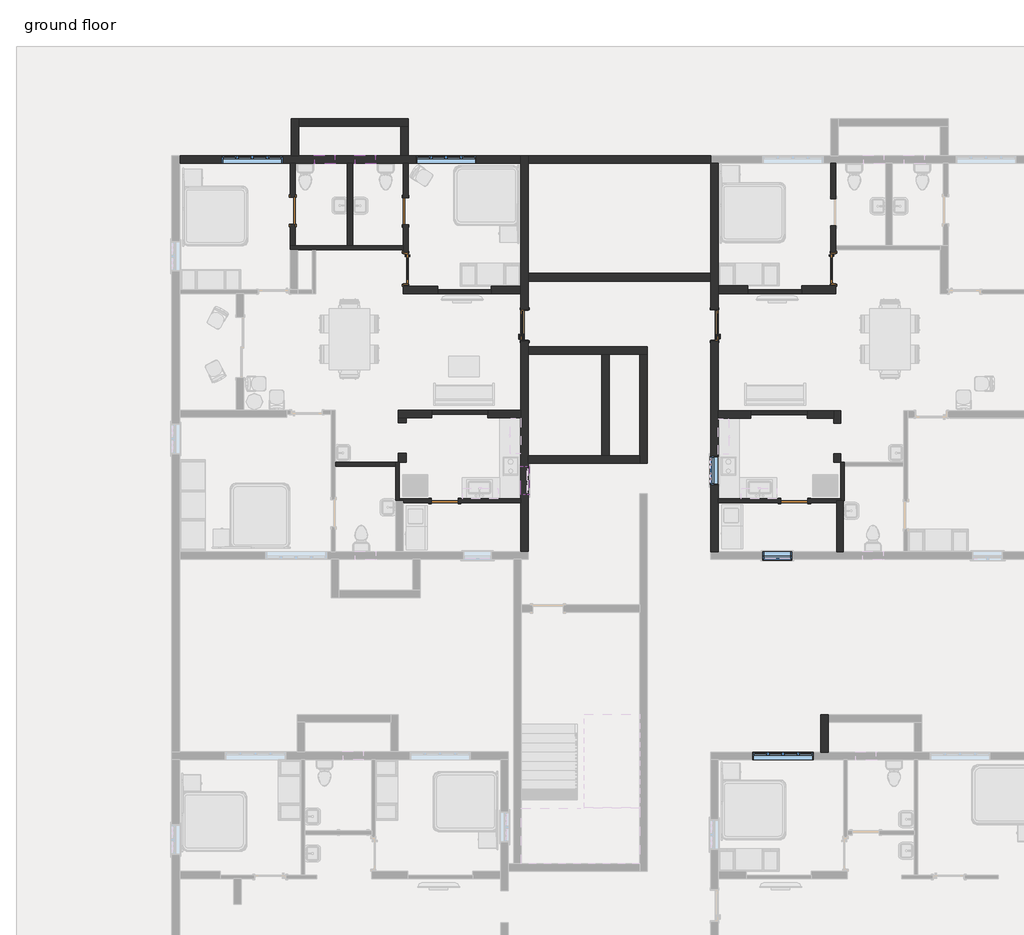
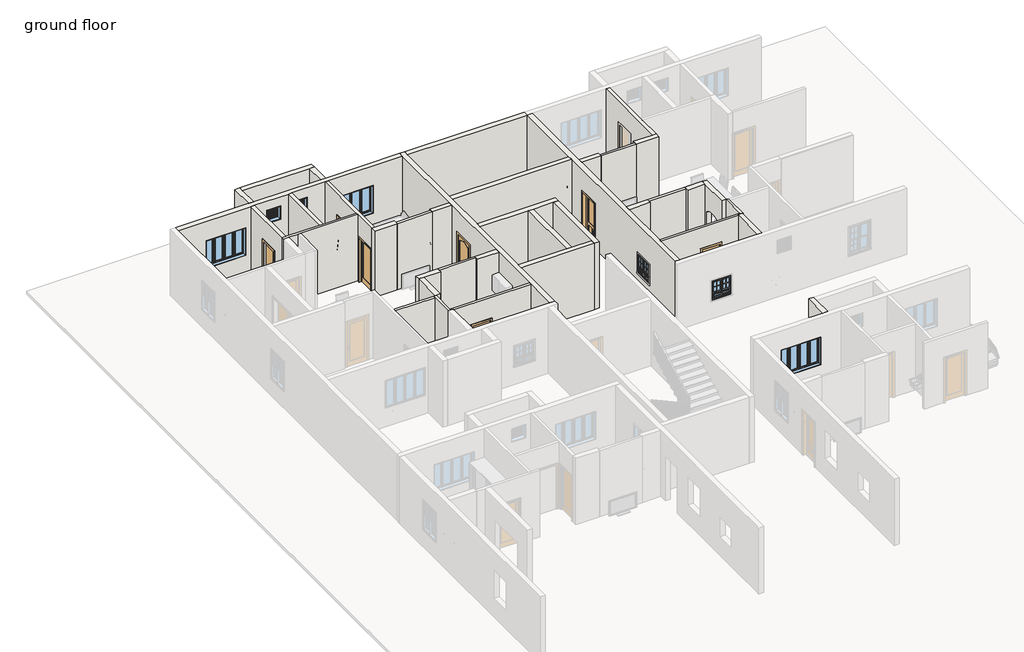
# One storey, part 8 of 16: 38 walls, 8 doors, 8 windows.
"""IFC4 building model written with IfcOpenShell, lengths in millimetres."""

from ifc_helpers import new_model, si_unit, point, frame, origin, place, context, project, spatial, polyline, ellipse_curve, trimmed, outline, extrude, faceted_brep, transform, mapped, element, save
from ifc_brep_helpers import plane_surface, extruded_surface, advanced_brep
from components import door_fe8ae985, door_f079f64e, door_010cc4d9, door_5a860750, door_377e7377, door_bb092f7c, door_38851409, door_d141acb4, window_ced37e8f, window_5487fb6d, window_f2d8fef0

model = new_model("IFC4")

# Units and contexts
model_context = context("Model", 3, world=origin())
ifc_project = project(units=[si_unit("LENGTHUNIT", "METRE", prefix="MILLI")], contexts=[model_context])

# Site, building, storey
site = spatial("IfcSite", under=ifc_project)
building = spatial("IfcBuilding", under=site)
storey = spatial("IfcBuildingStorey", under=building, Name="ground floor", Elevation=609.6)

# Doors
placement = place(None, origin())
door_shape = door_fe8ae985(model_context)
element("IfcDoor", 1, ObjectType="36\" x 84\"", at=placement, inside=storey, context=model_context, shape_type="MappedRepresentation", body=[
    mapped(door_shape, transform((53752.6562819, 45481.1632967, 609.6), x_axis=(0.0, -1.0, 0.0), y_axis=(1.0, 0.0, 0.0), z_axis=(0.0, 0.0, 1.0))),
])
door_2_shape = door_f079f64e(model_context)
element("IfcDoor", 2, ObjectType="36\" x 84\"", at=placement, inside=storey, context=model_context, shape_type="MappedRepresentation", body=[
    mapped(door_2_shape, transform((59474.0062819, 45484.6897902, 609.6), x_axis=(0.0, -1.0, 0.0), y_axis=(1.0, 0.0, 0.0), z_axis=(0.0, 0.0, 1.0))),
])
door_3_shape = door_010cc4d9(model_context)
element("IfcDoor", 3, ObjectType="Door-Interior-Single-1_Panel-Wood : 36\" x 84\"", at=placement, inside=storey, context=model_context, shape_type="MappedRepresentation", body=[
    mapped(door_3_shape, transform((50176.2761467, 47182.1953111, 609.6), x_axis=(0.0, -1.0, 0.0), y_axis=(1.0, 0.0, 0.0), z_axis=(0.0, 0.0, 1.0))),
])
door_4_shape = door_5a860750(model_context)
element("IfcDoor", 4, ObjectType="Door-Interior-Single-1_Panel-Wood : 36\" x 84\"", at=placement, inside=storey, context=model_context, shape_type="MappedRepresentation", body=[
    mapped(door_4_shape, transform((63047.8961425, 47183.9585579, 609.6), x_axis=(0.0, -1.0, 0.0), y_axis=(1.0, 0.0, 0.0), z_axis=(0.0, 0.0, 1.0))),
])
door_5_shape = door_377e7377(model_context)
element("IfcDoor", 5, ObjectType="Single-Flush : 32\" x 84\"", at=placement, inside=storey, context=model_context, shape_type="MappedRepresentation", body=[
    mapped(door_5_shape, transform((46777.7808276, 48934.0273256, 609.6), x_axis=(0.0, -1.0, 0.0), y_axis=(1.0, 0.0, 0.0), z_axis=(0.0, 0.0, 1.0))),
])
door_6_shape = door_bb092f7c(model_context)
element("IfcDoor", 6, ObjectType="Single-Flush : 32\" x 84\"", at=placement, inside=storey, context=model_context, shape_type="MappedRepresentation", body=[
    mapped(door_6_shape, transform((50173.1011467, 48908.6273256, 609.6), x_axis=(0.0, -1.0, 0.0), y_axis=(1.0, 0.0, 0.0), z_axis=(0.0, 0.0, 1.0))),
])
door_7_shape = door_38851409(model_context)
element("IfcDoor", 7, ObjectType="Single-Flush : 32\" x 84\"", at=placement, inside=storey, context=model_context, shape_type="MappedRepresentation", body=[
    mapped(door_7_shape, transform((61878.3731635, 40199.4543028, 609.6), x_axis=(1.0, 0.0, 0.0), y_axis=(0.0, 1.0, 0.0), z_axis=(0.0, 0.0, 1.0))),
])
door_8_shape = door_d141acb4(model_context)
element("IfcDoor", 8, ObjectType="Single-Flush : 32\" x 84\"", at=placement, inside=storey, context=model_context, shape_type="MappedRepresentation", body=[
    mapped(door_8_shape, transform((51357.158718, 40199.4543028, 609.6), x_axis=(-1.0, 0.0, 0.0), y_axis=(0.0, -1.0, 0.0), z_axis=(0.0, 0.0, 1.0))),
])

# Walls
element("IfcWall", 9, ObjectType="Generic - 4.5\"", at=placement, inside=storey, context=model_context, shape_type="SweptSolid", body=[
    extrude(outline(polyline([(51136.055056, 46547.9632967), (52747.8718849, 46547.9632967), (52747.8718849, 46433.6632967), (51136.055056, 46433.6632967), (51136.055056, 46547.9632967)])), frame((0.0, 0.0, 609.6), z_axis=(0.0, 0.0, 1.0), x_axis=(1.0, 0.0, 0.0)), (0.0, 0.0, 1.0), 3200.4),
])
element("IfcWall", 10, ObjectType="Generic - 4.5\"", at=placement, inside=storey, context=model_context, shape_type="SweptSolid", body=[
    extrude(outline(polyline([(50962.7840566, 42923.39304), (52649.6172737, 42923.39304), (52649.6172737, 42809.09304), (50962.7840566, 42809.09304), (50962.7840566, 42923.39304)])), frame((0.0, 0.0, 609.6), z_axis=(0.0, 0.0, 1.0), x_axis=(1.0, 0.0, 0.0)), (0.0, 0.0, 1.0), 3200.4),
])
element("IfcWall", 11, ObjectType="Generic - 4.5\"", at=placement, inside=storey, context=model_context, shape_type="Brep", body=[
    faceted_brep([(49985.558718, 40199.4543028, 609.6), (49985.558718, 40256.6043028, 609.6), (49985.558718, 41357.9395295, 609.6), (49985.558718, 41357.9395295, 3810.0), (49985.558718, 40256.6043028, 3810.0), (49985.558718, 40199.4543028, 3810.0), (49871.258718, 40199.4543028, 609.6), (49871.258718, 40199.4543028, 3810.0), (49871.258718, 41243.6395295, 3810.0), (49871.258718, 41357.9395295, 3810.0), (49871.258718, 41357.9395295, 609.6), (49871.258718, 41243.6395295, 609.6), (49958.6149004, 41357.9395295, 609.6), (49958.6149004, 41357.9395295, 3810.0)], [[[0, 1, 2, 3, 4, 5]], [[6, 7, 8, 9, 10, 11]], [[2, 1, 0, 6, 11, 10, 12]], [[5, 4, 3, 13, 9, 8, 7]], [[0, 5, 7, 6]], [[3, 2, 12, 10, 9, 13]]]),
])
element("IfcWall", 12, ObjectType="Generic - 4.5\"", at=placement, inside=storey, context=model_context, shape_type="SweptSolid", body=[
    extrude(outline(polyline([(48055.4368314, 41357.9395295), (49871.258718, 41357.9395295), (49871.258718, 41243.6395295), (48055.4368314, 41243.6395295), (48055.4368314, 41357.9395295)])), frame((0.0, 0.0, 609.6), z_axis=(0.0, 0.0, 1.0), x_axis=(1.0, 0.0, 0.0)), (0.0, 0.0, 1.0), 3200.4),
])
element("IfcWall", 13, ObjectType="Generic - 4.5\"", at=placement, inside=storey, context=model_context, shape_type="Brep", body=[
    faceted_brep([(50950.758718, 40256.6043028, 2743.2), (50950.758718, 40256.6043028, 609.6), (49985.558718, 40256.6043028, 609.6), (49985.558718, 40256.6043028, 3810.0), (53641.5312819, 40256.6043028, 3810.0), (53641.5312819, 40256.6043028, 609.6), (51763.558718, 40256.6043028, 609.6), (51763.558718, 40256.6043028, 2743.2), (50099.858718, 40142.3043028, 609.6), (50950.758718, 40142.3043028, 609.6), (50950.758718, 40142.3043028, 2743.2), (51763.558718, 40142.3043028, 2743.2), (51763.558718, 40142.3043028, 609.6), (53641.5312819, 40142.3043028, 609.6), (53641.5312819, 40142.3043028, 3810.0), (50099.858718, 40142.3043028, 3810.0), (50099.858718, 40199.4543028, 609.6), (49985.558718, 40199.4543028, 609.6), (49985.558718, 40199.4543028, 3810.0), (50099.858718, 40199.4543028, 3810.0)], [[[0, 1, 2, 3, 4, 5, 6, 7]], [[8, 9, 10, 11, 12, 13, 14, 15]], [[6, 5, 13, 12]], [[2, 1, 9, 8, 16, 17]], [[4, 3, 18, 19, 15, 14]], [[3, 2, 17, 18]], [[17, 16, 19, 18]], [[16, 8, 15, 19]], [[5, 4, 14, 13]], [[10, 9, 1, 0]], [[11, 10, 0, 7]], [[12, 11, 7, 6]]]),
])
element("IfcWall", 14, ObjectType="Generic - 4.5\"", at=placement, inside=storey, context=model_context, shape_type="Brep", body=[
    faceted_brep([(46701.6837344, 47759.2773256, 609.6), (46930.2837344, 47759.2773256, 609.6), (47362.0837344, 47759.2773256, 609.6), (47476.3837344, 47759.2773256, 609.6), (50096.9011467, 47759.2773256, 609.6), (50096.9011467, 47759.2773256, 3810.0), (47476.3837344, 47759.2773256, 3810.0), (47362.0837344, 47759.2773256, 3810.0), (46930.2837344, 47759.2773256, 3810.0), (46701.6837344, 47759.2773256, 3810.0), (46701.6837344, 47873.5773256, 609.6), (46701.6837344, 47873.5773256, 3810.0), (46853.9808276, 47873.5773256, 3810.0), (48424.8643084, 47873.5773256, 3810.0), (48577.2643084, 47873.5773256, 3810.0), (50096.9011467, 47873.5773256, 3810.0), (50096.9011467, 47873.5773256, 609.6), (48577.2643084, 47873.5773256, 609.6), (48424.8643084, 47873.5773256, 609.6), (46853.9808276, 47873.5773256, 609.6)], [[[0, 1, 2, 3, 4, 5, 6, 7, 8, 9]], [[10, 11, 12, 13, 14, 15, 16, 17, 18, 19]], [[4, 3, 2, 1, 0, 10, 19, 18, 17, 16]], [[9, 8, 7, 6, 5, 15, 14, 13, 12, 11]], [[0, 9, 11, 10]], [[5, 4, 16, 15]]]),
])
element("IfcWall", 15, ObjectType="Generic - 4.5\"", at=placement, inside=storey, context=model_context, shape_type="Brep", body=[
    faceted_brep([(63268.0476633, 41357.9395295, 609.6), (63268.0476633, 40256.6043028, 609.6), (63268.0476633, 40199.4543028, 609.6), (63268.0476633, 40199.4543028, 3810.0), (63268.0476633, 40256.6043028, 3810.0), (63268.0476633, 41357.9395295, 3810.0), (63382.3476633, 41357.9395295, 609.6), (63382.3476633, 41357.9395295, 3810.0), (63382.3476633, 41243.6395295, 3810.0), (63382.3476633, 40199.4543028, 3810.0), (63382.3476633, 40199.4543028, 609.6), (63382.3476633, 41243.6395295, 609.6), (63351.5731635, 40199.4543028, 609.6), (63351.5731635, 40199.4543028, 3810.0)], [[[0, 1, 2, 3, 4, 5]], [[6, 7, 8, 9, 10, 11]], [[2, 1, 0, 6, 11, 10, 12]], [[3, 2, 12, 10, 9, 13]], [[5, 4, 3, 13, 9, 8, 7]], [[0, 5, 7, 6]]]),
])
element("IfcWall", 16, ObjectType="Generic - 4.5\"", at=placement, inside=storey, context=model_context, shape_type="Brep", body=[
    faceted_brep([(62284.7731635, 40142.3043028, 2743.2), (62284.7731635, 40142.3043028, 609.6), (63148.3731635, 40142.3043028, 609.6), (63148.3731635, 40142.3043028, 3810.0), (59585.1312819, 40142.3043028, 3810.0), (59585.1312819, 40142.3043028, 609.6), (61471.9731635, 40142.3043028, 609.6), (61471.9731635, 40142.3043028, 2743.2), (63268.0476633, 40256.6043028, 609.6), (62284.7731635, 40256.6043028, 609.6), (62284.7731635, 40256.6043028, 2743.2), (61471.9731635, 40256.6043028, 2743.2), (61471.9731635, 40256.6043028, 609.6), (59585.1312819, 40256.6043028, 609.6), (59585.1312819, 40256.6043028, 3810.0), (63268.0476633, 40256.6043028, 3810.0), (63268.0476633, 40199.4543028, 609.6), (63148.3731635, 40199.4543028, 609.6), (63148.3731635, 40199.4543028, 3810.0), (63268.0476633, 40199.4543028, 3810.0)], [[[0, 1, 2, 3, 4, 5, 6, 7]], [[8, 9, 10, 11, 12, 13, 14, 15]], [[6, 5, 13, 12]], [[2, 1, 9, 8, 16, 17]], [[4, 3, 18, 19, 15, 14]], [[3, 2, 17, 18]], [[17, 16, 19, 18]], [[16, 8, 15, 19]], [[5, 4, 14, 13]], [[10, 9, 1, 0]], [[11, 10, 0, 7]], [[12, 11, 7, 6]]]),
])
element("IfcWall", 17, ObjectType="Generic - 4.5\"", at=placement, inside=storey, context=model_context, shape_type="SweptSolid", body=[
    extrude(outline(polyline([(62264.8312819, 42791.3797667), (60563.0312819, 42791.3797667), (60563.0312819, 42905.6797667), (62264.8312819, 42905.6797667), (62264.8312819, 42791.3797667)])), frame((0.0, 0.0, 609.6), z_axis=(0.0, 0.0, 1.0), x_axis=(1.0, 0.0, 0.0)), (0.0, 0.0, 1.0), 3200.4),
])
element("IfcWall", 18, ObjectType="Generic - 4.5\"", at=placement, inside=storey, context=model_context, shape_type="SweptSolid", body=[
    extrude(outline(polyline([(60478.7906788, 46551.4897902), (62090.6075077, 46551.4897902), (62090.6075077, 46437.1897902), (60478.7906788, 46437.1897902), (60478.7906788, 46551.4897902)])), frame((0.0, 0.0, 609.6), z_axis=(0.0, 0.0, 1.0), x_axis=(1.0, 0.0, 0.0)), (0.0, 0.0, 1.0), 3200.4),
])
element("IfcWall", 19, ObjectType="Generic - 6\"", at=placement, inside=storey, context=model_context, shape_type="SweptSolid", body=[
    extrude(outline(polyline([(48527.6273256, 2743.2), (48527.6273256, 609.6), (47873.5773256, 609.6), (47873.5773256, 3810.0), (50354.4390836, 3810.0), (50354.4390836, 609.6), (49340.4273256, 609.6), (49340.4273256, 2743.2), (48527.6273256, 2743.2)])), frame((46701.5808276, 0.0, 0.0), z_axis=(1.0, 0.0, 0.0), x_axis=(0.0, 1.0, 0.0)), (0.0, 0.0, 1.0), 152.4),
])
element("IfcWall", 20, ObjectType="Generic - 6\"", at=placement, inside=storey, context=model_context, shape_type="SweptSolid", body=[
    extrude(outline(polyline([(48424.8643084, 47873.5773256), (48424.8643084, 50354.4390836), (48577.2643084, 50354.4390836), (48577.2643084, 47873.5773256), (48424.8643084, 47873.5773256)])), frame((0.0, 0.0, 609.6), z_axis=(0.0, 0.0, 1.0), x_axis=(1.0, 0.0, 0.0)), (0.0, 0.0, 1.0), 3200.4),
])
element("IfcWall", 21, ObjectType="Generic - 6\"", at=placement, inside=storey, context=model_context, shape_type="Brep", body=[
    faceted_brep([(50096.9011467, 46662.2632967, 3810.0), (50096.9011467, 47759.2773256, 3810.0), (50096.9011467, 47873.5773256, 3810.0), (50096.9011467, 50354.4390836, 3810.0), (50096.9011467, 50354.4390836, 609.6), (50096.9011467, 49315.0273256, 609.6), (50096.9011467, 49315.0273256, 2743.2), (50096.9011467, 48502.2273256, 2743.2), (50096.9011467, 48502.2273256, 609.6), (50096.9011467, 47873.5773256, 609.6), (50096.9011467, 47759.2773256, 609.6), (50096.9011467, 47664.7953111, 609.6), (50096.9011467, 47664.7953111, 2768.6), (50096.9011467, 46699.5953111, 2768.6), (50096.9011467, 46699.5953111, 609.6), (50096.9011467, 46662.2632967, 609.6), (50249.3011467, 50354.4390836, 3810.0), (50249.3011467, 46662.2632967, 3810.0), (50249.3011467, 46662.2632967, 609.6), (50249.3011467, 46699.5953111, 609.6), (50249.3011467, 46699.5953111, 2768.6), (50249.3011467, 47664.7953111, 2768.6), (50249.3011467, 47664.7953111, 609.6), (50249.3011467, 48502.2273256, 609.6), (50249.3011467, 48502.2273256, 2743.2), (50249.3011467, 49315.0273256, 2743.2), (50249.3011467, 49315.0273256, 609.6), (50249.3011467, 50354.4390836, 609.6)], [[[0, 1, 2, 3, 4, 5, 6, 7, 8, 9, 10, 11, 12, 13, 14, 15]], [[16, 17, 18, 19, 20, 21, 22, 23, 24, 25, 26, 27]], [[4, 27, 26, 5]], [[18, 15, 14, 19]], [[8, 23, 22, 11, 10, 9]], [[3, 2, 1, 0, 17, 16]], [[4, 3, 16, 27]], [[0, 15, 18, 17]], [[24, 23, 8, 7]], [[25, 24, 7, 6]], [[26, 25, 6, 5]], [[13, 20, 19, 14]], [[20, 13, 12, 21]], [[21, 12, 11, 22]]]),
])
element("IfcWall", 22, ObjectType="Generic - 6\"", at=placement, inside=storey, context=model_context, shape_type="Brep", body=[
    faceted_brep([(62974.8711425, 48476.8273256, 2743.2), (62974.8711425, 48476.8273256, 609.6), (62974.8711425, 47666.5585579, 609.6), (62974.8711425, 47666.5585579, 2768.6), (62974.8711425, 46701.3585579, 2768.6), (62974.8711425, 46701.3585579, 609.6), (62974.8711425, 46665.7897902, 609.6), (62974.8711425, 46665.7897902, 3810.0), (62974.8711425, 50354.4390836, 3810.0), (62974.8711425, 50354.4390836, 609.6), (62974.8711425, 49289.6273256, 609.6), (62974.8711425, 49289.6273256, 2743.2), (63127.2711425, 47666.5585579, 609.6), (63127.2711425, 47759.2773256, 609.6), (63127.2711425, 47873.5773256, 609.6), (63127.2711425, 48476.8273256, 609.6), (63127.2711425, 48476.8273256, 2743.2), (63127.2711425, 49289.6273256, 2743.2), (63127.2711425, 49289.6273256, 609.6), (63127.2711425, 50354.4390836, 609.6), (63127.2711425, 50354.4390836, 3810.0), (63127.2711425, 47873.5773256, 3810.0), (63127.2711425, 47759.2773256, 3810.0), (63127.2711425, 46665.7897902, 3810.0), (63127.2711425, 46665.7897902, 609.6), (63127.2711425, 46701.3585579, 609.6), (63127.2711425, 46701.3585579, 2768.6), (63127.2711425, 47666.5585579, 2768.6)], [[[0, 1, 2, 3, 4, 5, 6, 7, 8, 9, 10, 11]], [[12, 13, 14, 15, 16, 17, 18, 19, 20, 21, 22, 23, 24, 25, 26, 27]], [[24, 6, 5, 25]], [[10, 9, 19, 18]], [[2, 1, 15, 14, 13, 12]], [[8, 7, 23, 22, 21, 20]], [[7, 6, 24, 23]], [[9, 8, 20, 19]], [[4, 26, 25, 5]], [[26, 4, 3, 27]], [[27, 3, 2, 12]], [[16, 15, 1, 0]], [[17, 16, 0, 11]], [[18, 17, 11, 10]]]),
])
element("IfcWall", 23, ObjectType="Generic - 8\"", at=placement, inside=storey, context=model_context, shape_type="AdvancedBrep", body=[
    advanced_brep(
    [(63064.8476633, 42905.6797667, 609.6), (63064.8476633, 42677.0797667, 609.6), (63064.8476633, 42531.8596481, 609.6), (63064.8476633, 42531.8596481, 2540.0), (63064.8476633, 41617.4596481, 2540.0), (63064.8476633, 41617.4596481, 609.6), (63064.8476633, 41357.9395295, 609.6), (63064.8476633, 41357.9395295, 3810.0), (63064.8476633, 42677.0797667, 3810.0), (63064.8476633, 42905.6797667, 3810.0), (63268.0476633, 42531.8596481, 2540.0), (63268.0476633, 42531.8596481, 609.6), (63268.0476633, 42905.6797667, 609.6), (63268.0476633, 42905.6797667, 3810.0), (63268.0476633, 41357.9395295, 3810.0), (63268.0476633, 41357.9395295, 609.6), (63268.0476633, 41617.4596481, 609.6), (63268.0476633, 41617.4596481, 2540.0)],
    [
        (0, 1),
        (1, 2),
        (2, 3),
        (3, 4, ellipse_curve(frame((63064.8476633, 42074.6596481, 2540.0), z_axis=(1.0, 0.0, 0.0), x_axis=(0.0, 1.0, 0.0)), 457.2, 203.2)),
        (4, 5),
        (5, 6),
        (6, 7),
        (7, 8),
        (8, 9),
        (9, 0),
        (10, 11),
        (11, 12),
        (12, 13),
        (13, 14),
        (14, 15),
        (15, 16),
        (16, 17),
        (17, 10, ellipse_curve(frame((63268.0476633, 42074.6596481, 2540.0), z_axis=(-1.0, 0.0, 0.0), x_axis=(0.0, 1.0, 0.0)), 457.2, 203.2)),
        (15, 6),
        (5, 16),
        (11, 2),
        (0, 12),
        (14, 7),
        (13, 9),
        (3, 10),
        (17, 4),
    ],
    [
        plane_surface(frame((63064.8476633, 42694.79304, 609.6), z_axis=(-1.0, 0.0, 0.0), x_axis=(0.0, -1.0, 0.0))),
        plane_surface(frame((63268.0476633, 42694.79304, 609.6), z_axis=(1.0, 0.0, 0.0), x_axis=(0.0, 1.0, 0.0))),
        plane_surface(frame((63064.8476633, 42791.3797667, 609.6), z_axis=(0.0, 0.0, -1.0), x_axis=(1.0, 0.0, 0.0))),
        plane_surface(frame((63064.8476633, 41357.9395295, 609.6), z_axis=(0.0, -1.0, 0.0), x_axis=(1.0, 0.0, 0.0))),
        plane_surface(frame((63064.8476633, 41357.9395295, 3810.0), z_axis=(0.0, 0.0, 1.0), x_axis=(1.0, 0.0, 0.0))),
        plane_surface(frame((63239.9057173, 42905.6797667, 609.6), z_axis=(0.0, 1.0, 0.0), x_axis=(-1.0, 0.0, 0.0))),
        extruded_surface(trimmed(ellipse_curve(frame((63471.2476633, 42074.6596481, 2540.0), z_axis=(1.0, 0.0, 0.0), x_axis=(0.0, 1.0, 0.0)), 457.2, 203.2), [point((63471.2476633, 42531.8596481, 2540.0))], [point((63471.2476633, 41617.4596481, 2540.0))], True, "CARTESIAN"), (-203.1999999999971, 0.0, 0.0), 203.1999999999971),
        plane_surface(frame((63064.8476633, 41617.4596481, 2540.0), z_axis=(0.0, 1.0, 0.0), x_axis=(1.0, 0.0, 0.0))),
        plane_surface(frame((63064.8476633, 42531.8596481, 609.6), z_axis=(0.0, -1.0, 0.0), x_axis=(1.0, 0.0, 0.0))),
    ],
    [
        (0, [[1, 2, 3, 4, 5, 6, 7, 8, 9, 10]]),
        (1, [[11, 12, 13, 14, 15, 16, 17, 18]]),
        (2, [[-16, 19, -6, 20]]),
        (2, [[-12, 21, -2, -1, 22]]),
        (3, [[-7, -19, -15, 23]]),
        (4, [[-9, -8, -23, -14, 24]]),
        (5, [[-10, -24, -13, -22]]),
        (6, [[-4, 25, -18, 26]]),
        (7, [[-5, -26, -17, -20]]),
        (8, [[-3, -21, -11, -25]]),
    ],
),
])
element("IfcWall", 24, ObjectType="Generic - 8\"", at=placement, inside=storey, context=model_context, shape_type="Brep", body=[
    faceted_brep([(63351.5731635, 38662.1809867, 609.6), (63351.5731635, 40199.4543028, 609.6), (63351.5731635, 40199.4543028, 3810.0), (63351.5731635, 38662.1809867, 3810.0), (63148.3731635, 38662.1809867, 609.6), (63148.3731635, 38662.1809867, 3810.0), (63148.3731635, 40142.3043028, 3810.0), (63148.3731635, 40199.4543028, 3810.0), (63148.3731635, 40199.4543028, 609.6), (63148.3731635, 40142.3043028, 609.6), (63268.0476633, 40199.4543028, 609.6), (63268.0476633, 40199.4543028, 3810.0)], [[[0, 1, 2, 3]], [[4, 5, 6, 7, 8, 9]], [[1, 0, 4, 9, 8, 10]], [[2, 1, 10, 8, 7, 11]], [[3, 2, 11, 7, 6, 5]], [[0, 3, 5, 4]]]),
])
element("IfcWall", 25, ObjectType="Generic - 9\"", at=placement, inside=storey, context=model_context, shape_type="Brep", body=[
    faceted_brep([(53870.1312819, 50583.0390836, 3810.0), (53870.1312819, 50354.4390836, 3810.0), (53870.1312819, 47041.6375431, 3810.0), (53870.1312819, 46813.0375431, 3810.0), (53870.1312819, 44831.8375431, 3810.0), (53870.1312819, 44603.2375431, 3810.0), (53870.1312819, 41555.2375431, 3810.0), (53870.1312819, 41326.6375431, 3810.0), (53870.1312819, 38662.1809867, 3810.0), (53870.1312819, 38662.1809867, 609.6), (53870.1312819, 41326.6375431, 609.6), (53870.1312819, 41555.2375431, 609.6), (53870.1312819, 44603.2375431, 609.6), (53870.1312819, 44831.8375431, 609.6), (53870.1312819, 44998.5632967, 609.6), (53870.1312819, 44998.5632967, 2768.6), (53870.1312819, 45963.7632967, 2768.6), (53870.1312819, 45963.7632967, 609.6), (53870.1312819, 46813.0375431, 609.6), (53870.1312819, 47041.6375431, 609.6), (53870.1312819, 50354.4390836, 609.6), (53870.1312819, 50583.0390836, 609.6), (53870.1312819, 40377.2543028, 2743.2), (53870.1312819, 41240.8543028, 2743.2), (53870.1312819, 41240.8543028, 1828.8), (53870.1312819, 40377.2543028, 1828.8), (53641.5312819, 38662.1809867, 3810.0), (53641.5312819, 40142.3043028, 3810.0), (53641.5312819, 40256.6043028, 3810.0), (53641.5312819, 42694.79304, 3810.0), (53641.5312819, 42923.39304, 3810.0), (53641.5312819, 46433.6632967, 3810.0), (53641.5312819, 46662.2632967, 3810.0), (53641.5312819, 50354.4390836, 3810.0), (53641.5312819, 50583.0390836, 3810.0), (53641.5312819, 50583.0390836, 609.6), (53641.5312819, 50354.4390836, 609.6), (53641.5312819, 46662.2632967, 609.6), (53641.5312819, 46433.6632967, 609.6), (53641.5312819, 45963.7632967, 609.6), (53641.5312819, 45963.7632967, 2768.6), (53641.5312819, 44998.5632967, 2768.6), (53641.5312819, 44998.5632967, 609.6), (53641.5312819, 42923.39304, 609.6), (53641.5312819, 42694.79304, 609.6), (53641.5312819, 40256.6043028, 609.6), (53641.5312819, 40142.3043028, 609.6), (53641.5312819, 38662.1809867, 609.6), (53641.5312819, 40377.2543028, 2743.2), (53641.5312819, 40377.2543028, 1828.8), (53641.5312819, 41240.8543028, 1828.8), (53641.5312819, 41240.8543028, 2743.2)], [[[0, 1, 2, 3, 4, 5, 6, 7, 8, 9, 10, 11, 12, 13, 14, 15, 16, 17, 18, 19, 20, 21], [22, 23, 24, 25]], [[26, 27, 28, 29, 30, 31, 32, 33, 34, 35, 36, 37, 38, 39, 40, 41, 42, 43, 44, 45, 46, 47], [48, 49, 50, 51]], [[9, 47, 46, 45, 44, 43, 42, 14, 13, 12, 11, 10]], [[35, 21, 20, 19, 18, 17, 39, 38, 37, 36]], [[8, 7, 6, 5, 4, 3, 2, 1, 0, 34, 33, 32, 31, 30, 29, 28, 27, 26]], [[9, 8, 26, 47]], [[0, 21, 35, 34]], [[49, 48, 22, 25]], [[50, 49, 25, 24]], [[51, 50, 24, 23]], [[48, 51, 23, 22]], [[41, 15, 14, 42]], [[15, 41, 40, 16]], [[16, 40, 39, 17]]]),
])
element("IfcWall", 26, ObjectType="Generic - 9\"", at=placement, inside=storey, context=model_context, shape_type="Brep", body=[
    faceted_brep([(53641.5312819, 50583.0390836, 609.6), (50249.3011467, 50583.0390836, 609.6), (50020.7011467, 50583.0390836, 609.6), (46954.5399066, 50583.0390836, 609.6), (46725.9399066, 50583.0390836, 609.6), (43370.226243, 50583.0390836, 609.6), (43370.226243, 50583.0390836, 3810.0), (46725.9399066, 50583.0390836, 3810.0), (46954.5399066, 50583.0390836, 3810.0), (50020.7011467, 50583.0390836, 3810.0), (50249.3011467, 50583.0390836, 3810.0), (53641.5312819, 50583.0390836, 3810.0), (47434.2643084, 50583.0390836, 3352.8), (47434.2643084, 50583.0390836, 2743.2), (48043.8643084, 50583.0390836, 2743.2), (48043.8643084, 50583.0390836, 3352.8), (48653.4643084, 50583.0390836, 3352.8), (48653.4643084, 50583.0390836, 2743.2), (49263.0643084, 50583.0390836, 2743.2), (49263.0643084, 50583.0390836, 3352.8), (46472.9808276, 50583.0390836, 2870.2), (44644.1808276, 50583.0390836, 2870.2), (44644.1808276, 50583.0390836, 1524.0), (46472.9808276, 50583.0390836, 1524.0), (52306.7011467, 50583.0390836, 2870.2), (50477.9011467, 50583.0390836, 2870.2), (50477.9011467, 50583.0390836, 1524.0), (52306.7011467, 50583.0390836, 1524.0), (53641.5312819, 50354.4390836, 609.6), (53641.5312819, 50354.4390836, 3810.0), (50249.3011467, 50354.4390836, 3810.0), (50096.9011467, 50354.4390836, 3810.0), (48577.2643084, 50354.4390836, 3810.0), (48424.8643084, 50354.4390836, 3810.0), (46853.9808276, 50354.4390836, 3810.0), (46701.5808276, 50354.4390836, 3810.0), (43370.226243, 50354.4390836, 3810.0), (43370.226243, 50354.4390836, 609.6), (46701.5808276, 50354.4390836, 609.6), (46853.9808276, 50354.4390836, 609.6), (48424.8643084, 50354.4390836, 609.6), (48577.2643084, 50354.4390836, 609.6), (50096.9011467, 50354.4390836, 609.6), (50249.3011467, 50354.4390836, 609.6), (47434.2643084, 50354.4390836, 3352.8), (48043.8643084, 50354.4390836, 3352.8), (48043.8643084, 50354.4390836, 2743.2), (47434.2643084, 50354.4390836, 2743.2), (48653.4643084, 50354.4390836, 3352.8), (49263.0643084, 50354.4390836, 3352.8), (49263.0643084, 50354.4390836, 2743.2), (48653.4643084, 50354.4390836, 2743.2), (46472.9808276, 50354.4390836, 2870.2), (46472.9808276, 50354.4390836, 1524.0), (44644.1808276, 50354.4390836, 1524.0), (44644.1808276, 50354.4390836, 2870.2), (52306.7011467, 50354.4390836, 2870.2), (52306.7011467, 50354.4390836, 1524.0), (50477.9011467, 50354.4390836, 1524.0), (50477.9011467, 50354.4390836, 2870.2)], [[[0, 1, 2, 3, 4, 5, 6, 7, 8, 9, 10, 11], [12, 13, 14, 15], [16, 17, 18, 19], [20, 21, 22, 23], [24, 25, 26, 27]], [[28, 29, 30, 31, 32, 33, 34, 35, 36, 37, 38, 39, 40, 41, 42, 43], [44, 45, 46, 47], [48, 49, 50, 51], [52, 53, 54, 55], [56, 57, 58, 59]], [[5, 4, 3, 2, 1, 0, 28, 43, 42, 41, 40, 39, 38, 37]], [[11, 10, 9, 8, 7, 6, 36, 35, 34, 33, 32, 31, 30, 29]], [[6, 5, 37, 36]], [[0, 11, 29, 28]], [[13, 12, 44, 47]], [[14, 13, 47, 46]], [[15, 14, 46, 45]], [[12, 15, 45, 44]], [[17, 16, 48, 51]], [[18, 17, 51, 50]], [[19, 18, 50, 49]], [[16, 19, 49, 48]], [[53, 52, 20, 23]], [[54, 53, 23, 22]], [[55, 54, 22, 21]], [[52, 55, 21, 20]], [[57, 56, 24, 27]], [[58, 57, 27, 26]], [[59, 58, 26, 25]], [[56, 59, 25, 24]]]),
])
element("IfcWall", 27, ObjectType="Generic - 9\"", at=placement, inside=storey, context=model_context, shape_type="Brep", body=[
    faceted_brep([(53641.5312819, 46662.2632967, 609.6), (52747.8718849, 46662.2632967, 609.6), (52747.8718849, 46662.2632967, 3810.0), (53641.5312819, 46662.2632967, 3810.0), (53641.5312819, 46433.6632967, 609.6), (53641.5312819, 46433.6632967, 3810.0), (52747.8718849, 46433.6632967, 3810.0), (52747.8718849, 46433.6632967, 609.6), (52747.8718849, 46547.9632967, 609.6), (52747.8718849, 46547.9632967, 3810.0)], [[[0, 1, 2, 3]], [[4, 5, 6, 7]], [[1, 0, 4, 7, 8]], [[2, 1, 8, 7, 6, 9]], [[3, 2, 9, 6, 5]], [[0, 3, 5, 4]]]),
])
element("IfcWall", 28, ObjectType="Generic - 9\"", at=placement, inside=storey, context=model_context, shape_type="Brep", body=[
    faceted_brep([(51136.055056, 46662.2632967, 609.6), (50249.3011467, 46662.2632967, 609.6), (50096.9011467, 46662.2632967, 609.6), (50096.9011467, 46662.2632967, 3810.0), (50249.3011467, 46662.2632967, 3810.0), (51136.055056, 46662.2632967, 3810.0), (51136.055056, 46433.6632967, 609.6), (51136.055056, 46433.6632967, 3810.0), (50096.9011467, 46433.6632967, 3810.0), (50096.9011467, 46433.6632967, 609.6), (51136.055056, 46547.9632967, 609.6), (51136.055056, 46547.9632967, 3810.0)], [[[0, 1, 2, 3, 4, 5]], [[6, 7, 8, 9]], [[2, 1, 0, 10, 6, 9]], [[5, 4, 3, 8, 7, 11]], [[0, 5, 11, 7, 6, 10]], [[3, 2, 9, 8]]]),
])
element("IfcWall", 29, ObjectType="Generic - 9\"", at=placement, inside=storey, context=model_context, shape_type="Brep", body=[
    faceted_brep([(53641.5312819, 42923.39304, 609.6), (52649.6172737, 42923.39304, 609.6), (52649.6172737, 42923.39304, 3810.0), (53641.5312819, 42923.39304, 3810.0), (53641.5312819, 42694.79304, 609.6), (53641.5312819, 42694.79304, 3810.0), (52649.6172737, 42694.79304, 3810.0), (52649.6172737, 42694.79304, 609.6), (52649.6172737, 42809.09304, 609.6), (52649.6172737, 42809.09304, 3810.0)], [[[0, 1, 2, 3]], [[4, 5, 6, 7]], [[1, 0, 4, 7, 8]], [[2, 1, 8, 7, 6, 9]], [[3, 2, 9, 6, 5]], [[0, 3, 5, 4]]]),
])
element("IfcWall", 30, ObjectType="Generic - 9\"", at=placement, inside=storey, context=model_context, shape_type="Brep", body=[
    faceted_brep([(50962.7840566, 42923.39304, 609.6), (49958.6149004, 42923.39304, 609.6), (49958.6149004, 42923.39304, 3810.0), (50962.7840566, 42923.39304, 3810.0), (50962.7840566, 42694.79304, 609.6), (50962.7840566, 42694.79304, 3810.0), (50187.2149004, 42694.79304, 3810.0), (49958.6149004, 42694.79304, 3810.0), (49958.6149004, 42694.79304, 609.6), (50187.2149004, 42694.79304, 609.6), (50962.7840566, 42809.09304, 609.6), (50962.7840566, 42809.09304, 3810.0)], [[[0, 1, 2, 3]], [[4, 5, 6, 7, 8, 9]], [[1, 0, 10, 4, 9, 8]], [[2, 1, 8, 7]], [[3, 2, 7, 6, 5, 11]], [[0, 3, 11, 5, 4, 10]]]),
])
element("IfcWall", 31, ObjectType="Generic - 9\"", at=placement, inside=storey, context=model_context, shape_type="AdvancedBrep", body=[
    advanced_brep(
    [(49958.6149004, 41626.3162847, 2540.0), (49958.6149004, 41626.3162847, 609.6), (49958.6149004, 41357.9395295, 609.6), (49958.6149004, 41357.9395295, 3810.0), (49958.6149004, 42694.79304, 3810.0), (49958.6149004, 42694.79304, 609.6), (49958.6149004, 42540.7162847, 609.6), (49958.6149004, 42540.7162847, 2540.0), (50187.2149004, 41357.9395295, 609.6), (50187.2149004, 41626.3162847, 609.6), (50187.2149004, 41626.3162847, 2540.0), (50187.2149004, 42540.7162847, 2540.0), (50187.2149004, 42540.7162847, 609.6), (50187.2149004, 42694.79304, 609.6), (50187.2149004, 42694.79304, 3810.0), (50187.2149004, 41357.9395295, 3810.0), (49985.558718, 41357.9395295, 609.6), (49985.558718, 41357.9395295, 3810.0)],
    [
        (0, 1),
        (1, 2),
        (2, 3),
        (3, 4),
        (4, 5),
        (5, 6),
        (6, 7),
        (7, 0, ellipse_curve(frame((49958.6149004, 42083.5162847, 2540.0), z_axis=(1.0, 0.0, 0.0), x_axis=(0.0, -1.0, 0.0)), 457.2, 203.2)),
        (8, 9),
        (9, 10),
        (10, 11, ellipse_curve(frame((50187.2149004, 42083.5162847, 2540.0), z_axis=(-1.0, 0.0, 0.0), x_axis=(0.0, -1.0, 0.0)), 457.2, 203.2)),
        (11, 12),
        (12, 13),
        (13, 14),
        (14, 15),
        (15, 8),
        (5, 13),
        (12, 6),
        (1, 9),
        (8, 16),
        (16, 2),
        (3, 17),
        (17, 15),
        (14, 4),
        (10, 0),
        (7, 11),
    ],
    [
        plane_surface(frame((49958.6149004, 42673.5469106, 609.6), z_axis=(-1.0, 0.0, 0.0), x_axis=(0.0, -1.0, 0.0))),
        plane_surface(frame((50187.2149004, 42673.5469106, 609.6), z_axis=(1.0, 0.0, 0.0), x_axis=(0.0, 1.0, 0.0))),
        plane_surface(frame((49958.6149004, 42809.09304, 609.6), z_axis=(0.0, 0.0, -1.0), x_axis=(1.0, 0.0, 0.0))),
        plane_surface(frame((49958.6149004, 41300.7895295, 3810.0), z_axis=(0.0, 0.0, 1.0), x_axis=(1.0, 0.0, 0.0))),
        plane_surface(frame((50962.7840566, 42694.79304, 609.6), z_axis=(0.0, 1.0, 0.0), x_axis=(1.0, 0.0, 0.0))),
        plane_surface(frame((49855.4911564, 41357.9395295, 609.6), z_axis=(0.0, -1.0, 0.0), x_axis=(-1.0, 0.0, 0.0))),
        extruded_surface(trimmed(ellipse_curve(frame((49730.0149004, 42083.5162847, 2540.0), z_axis=(-1.0, 0.0, 0.0), x_axis=(0.0, -1.0, 0.0)), 457.2, 203.2), [point((49730.0149004, 41626.3162847, 2540.0))], [point((49730.0149004, 42540.7162847, 2540.0))], True, "CARTESIAN"), (228.60000000000582, 0.0, 0.0), 228.60000000000582),
        plane_surface(frame((50187.2149004, 42540.7162847, 2540.0), z_axis=(0.0, -1.0, 0.0), x_axis=(-1.0, 0.0, 0.0))),
        plane_surface(frame((50187.2149004, 41626.3162847, 609.6), z_axis=(0.0, 1.0, 0.0), x_axis=(-1.0, 0.0, 0.0))),
    ],
    [
        (0, [[1, 2, 3, 4, 5, 6, 7, 8]]),
        (1, [[9, 10, 11, 12, 13, 14, 15, 16]]),
        (2, [[-6, 17, -13, 18]]),
        (2, [[-2, 19, -9, 20, 21]]),
        (3, [[-4, 22, 23, -15, 24]]),
        (4, [[-5, -24, -14, -17]]),
        (5, [[-3, -21, -20, -16, -23, -22]]),
        (6, [[-11, 25, -8, 26]]),
        (7, [[-12, -26, -7, -18]]),
        (8, [[-10, -19, -1, -25]]),
    ],
),
])
element("IfcWall", 32, ObjectType="Generic - 9\"", at=placement, inside=storey, context=model_context, shape_type="Brep", body=[
    faceted_brep([(46954.5399066, 50583.0390836, 609.6), (46954.5399066, 51470.3211687, 609.6), (46954.5399066, 51698.9211687, 609.6), (46954.5399066, 51698.9211687, 3810.0), (46954.5399066, 51470.3211687, 3810.0), (46954.5399066, 50583.0390836, 3810.0), (46725.9399066, 50583.0390836, 609.6), (46725.9399066, 50583.0390836, 3810.0), (46725.9399066, 51698.9211687, 3810.0), (46725.9399066, 51698.9211687, 609.6)], [[[0, 1, 2, 3, 4, 5]], [[6, 7, 8, 9]], [[2, 1, 0, 6, 9]], [[5, 4, 3, 8, 7]], [[0, 5, 7, 6]], [[3, 2, 9, 8]]]),
])
element("IfcWall", 33, ObjectType="Generic - 9\"", at=placement, inside=storey, context=model_context, shape_type="Brep", body=[
    faceted_brep([(46954.5399066, 51470.3211687, 609.6), (50020.7011467, 51470.3211687, 609.6), (50249.3011467, 51470.3211687, 609.6), (50249.3011467, 51470.3211687, 3810.0), (50020.7011467, 51470.3211687, 3810.0), (46954.5399066, 51470.3211687, 3810.0), (46954.5399066, 51698.9211687, 609.6), (46954.5399066, 51698.9211687, 3810.0), (50249.3011467, 51698.9211687, 3810.0), (50249.3011467, 51698.9211687, 609.6)], [[[0, 1, 2, 3, 4, 5]], [[6, 7, 8, 9]], [[2, 1, 0, 6, 9]], [[5, 4, 3, 8, 7]], [[0, 5, 7, 6]], [[3, 2, 9, 8]]]),
])
element("IfcWall", 34, ObjectType="Generic - 9\"", at=placement, inside=storey, context=model_context, shape_type="SweptSolid", body=[
    extrude(outline(polyline([(50020.7011467, 50583.0390836), (50020.7011467, 51470.3211687), (50249.3011467, 51470.3211687), (50249.3011467, 50583.0390836), (50020.7011467, 50583.0390836)])), frame((0.0, 0.0, 609.6), z_axis=(0.0, 0.0, 1.0), x_axis=(1.0, 0.0, 0.0)), (0.0, 0.0, 1.0), 3200.4),
])
element("IfcWall", 35, ObjectType="Generic - 9\"", at=placement, inside=storey, context=model_context, shape_type="Brep", body=[
    faceted_brep([(59585.1312819, 50354.4390836, 3810.0), (59585.1312819, 46665.7897902, 3810.0), (59585.1312819, 46437.1897902, 3810.0), (59585.1312819, 42905.6797667, 3810.0), (59585.1312819, 42677.0797667, 3810.0), (59585.1312819, 40256.6043028, 3810.0), (59585.1312819, 40142.3043028, 3810.0), (59585.1312819, 38662.1809867, 3810.0), (59585.1312819, 38662.1809867, 609.6), (59585.1312819, 40142.3043028, 609.6), (59585.1312819, 40256.6043028, 609.6), (59585.1312819, 42677.0797667, 609.6), (59585.1312819, 42905.6797667, 609.6), (59585.1312819, 45002.0897902, 609.6), (59585.1312819, 45002.0897902, 2768.6), (59585.1312819, 45967.2897902, 2768.6), (59585.1312819, 45967.2897902, 609.6), (59585.1312819, 46437.1897902, 609.6), (59585.1312819, 46665.7897902, 609.6), (59585.1312819, 50354.4390836, 609.6), (59585.1312819, 41545.6543028, 2438.4), (59585.1312819, 41545.6543028, 1524.0), (59585.1312819, 40682.0543028, 1524.0), (59585.1312819, 40682.0543028, 2438.4), (59356.5312819, 38662.1809867, 3810.0), (59356.5312819, 46813.0375431, 3810.0), (59356.5312819, 47041.6375431, 3810.0), (59356.5312819, 50354.4390836, 3810.0), (59356.5312819, 50354.4390836, 609.6), (59356.5312819, 47041.6375431, 609.6), (59356.5312819, 46813.0375431, 609.6), (59356.5312819, 45967.2897902, 609.6), (59356.5312819, 45967.2897902, 2768.6), (59356.5312819, 45002.0897902, 2768.6), (59356.5312819, 45002.0897902, 609.6), (59356.5312819, 38662.1809867, 609.6), (59356.5312819, 41545.6543028, 2438.4), (59356.5312819, 40682.0543028, 2438.4), (59356.5312819, 40682.0543028, 1524.0), (59356.5312819, 41545.6543028, 1524.0)], [[[0, 1, 2, 3, 4, 5, 6, 7, 8, 9, 10, 11, 12, 13, 14, 15, 16, 17, 18, 19], [20, 21, 22, 23]], [[24, 25, 26, 27, 28, 29, 30, 31, 32, 33, 34, 35], [36, 37, 38, 39]], [[8, 35, 34, 13, 12, 11, 10, 9]], [[28, 19, 18, 17, 16, 31, 30, 29]], [[7, 6, 5, 4, 3, 2, 1, 0, 27, 26, 25, 24]], [[0, 19, 28, 27]], [[8, 7, 24, 35]], [[33, 14, 13, 34]], [[14, 33, 32, 15]], [[15, 32, 31, 16]], [[21, 20, 36, 39]], [[22, 21, 39, 38]], [[23, 22, 38, 37]], [[20, 23, 37, 36]]]),
])
element("IfcWall", 36, ObjectType="Generic - 9\"", at=placement, inside=storey, context=model_context, shape_type="Brep", body=[
    faceted_brep([(59585.1312819, 46437.1897902, 609.6), (60478.7906788, 46437.1897902, 609.6), (60478.7906788, 46437.1897902, 3810.0), (59585.1312819, 46437.1897902, 3810.0), (59585.1312819, 46665.7897902, 609.6), (59585.1312819, 46665.7897902, 3810.0), (60478.7906788, 46665.7897902, 3810.0), (60478.7906788, 46665.7897902, 609.6), (60478.7906788, 46551.4897902, 609.6), (60478.7906788, 46551.4897902, 3810.0)], [[[0, 1, 2, 3]], [[4, 5, 6, 7]], [[1, 0, 4, 7, 8]], [[2, 1, 8, 7, 6, 9]], [[3, 2, 9, 6, 5]], [[0, 3, 5, 4]]]),
])
element("IfcWall", 37, ObjectType="Generic - 9\"", at=placement, inside=storey, context=model_context, shape_type="Brep", body=[
    faceted_brep([(62090.6075077, 46437.1897902, 609.6), (63127.2711425, 46437.1897902, 609.6), (63127.2711425, 46437.1897902, 3810.0), (62090.6075077, 46437.1897902, 3810.0), (62090.6075077, 46665.7897902, 609.6), (62090.6075077, 46665.7897902, 3810.0), (62974.8711425, 46665.7897902, 3810.0), (63127.2711425, 46665.7897902, 3810.0), (63127.2711425, 46665.7897902, 609.6), (62974.8711425, 46665.7897902, 609.6), (62090.6075077, 46551.4897902, 609.6), (62090.6075077, 46551.4897902, 3810.0)], [[[0, 1, 2, 3]], [[4, 5, 6, 7, 8, 9]], [[1, 0, 10, 4, 9, 8]], [[3, 2, 7, 6, 5, 11]], [[0, 3, 11, 5, 4, 10]], [[2, 1, 8, 7]]]),
])
element("IfcWall", 38, ObjectType="Generic - 9\"", at=placement, inside=storey, context=model_context, shape_type="Brep", body=[
    faceted_brep([(59585.1312819, 42677.0797667, 609.6), (60563.0312819, 42677.0797667, 609.6), (60563.0312819, 42677.0797667, 3810.0), (59585.1312819, 42677.0797667, 3810.0), (59585.1312819, 42905.6797667, 609.6), (59585.1312819, 42905.6797667, 3810.0), (60563.0312819, 42905.6797667, 3810.0), (60563.0312819, 42905.6797667, 609.6), (60563.0312819, 42791.3797667, 609.6), (60563.0312819, 42791.3797667, 3810.0)], [[[0, 1, 2, 3]], [[4, 5, 6, 7]], [[1, 0, 4, 7, 8]], [[2, 1, 8, 7, 6, 9]], [[3, 2, 9, 6, 5]], [[0, 3, 5, 4]]]),
])
element("IfcWall", 39, ObjectType="Generic - 9\"", at=placement, inside=storey, context=model_context, shape_type="Brep", body=[
    faceted_brep([(63064.8476633, 42905.6797667, 609.6), (62264.8312819, 42905.6797667, 609.6), (62264.8312819, 42905.6797667, 3810.0), (63064.8476633, 42905.6797667, 3810.0), (63064.8476633, 42677.0797667, 609.6), (63064.8476633, 42677.0797667, 3810.0), (62264.8312819, 42677.0797667, 3810.0), (62264.8312819, 42677.0797667, 609.6), (62264.8312819, 42791.3797667, 609.6), (62264.8312819, 42791.3797667, 3810.0)], [[[0, 1, 2, 3]], [[4, 5, 6, 7]], [[1, 0, 4, 7, 8]], [[2, 1, 8, 7, 6, 9]], [[3, 2, 9, 6, 5]], [[0, 3, 5, 4]]]),
])
element("IfcWall", 40, ObjectType="Generic - 9\"", at=placement, inside=storey, context=model_context, shape_type="Brep", body=[
    faceted_brep([(62892.3192161, 32628.9650652, 609.6), (62892.3192161, 33536.3470746, 609.6), (62892.3192161, 33764.9470746, 609.6), (62892.3192161, 33764.9470746, 3810.0), (62892.3192161, 33536.3470746, 3810.0), (62892.3192161, 32628.9650652, 3810.0), (62663.7192161, 32628.9650652, 609.6), (62663.7192161, 32628.9650652, 3810.0), (62663.7192161, 33764.9470746, 3810.0), (62663.7192161, 33764.9470746, 609.6)], [[[0, 1, 2, 3, 4, 5]], [[6, 7, 8, 9]], [[2, 1, 0, 6, 9]], [[5, 4, 3, 8, 7]], [[0, 5, 7, 6]], [[3, 2, 9, 8]]]),
])
element("IfcWall", 41, ObjectType="Generic - 9\"", at=placement, inside=storey, context=model_context, shape_type="SweptSolid", body=[
    extrude(outline(polyline([(59356.5312819, 50354.4390836), (53870.1312819, 50354.4390836), (53870.1312819, 50583.0390836), (59356.5312819, 50583.0390836), (59356.5312819, 50354.4390836)])), frame((0.0, 0.0, 609.6), z_axis=(0.0, 0.0, 1.0), x_axis=(1.0, 0.0, 0.0)), (0.0, 0.0, 1.0), 3200.4),
])
element("IfcWall", 42, ObjectType="Generic - 9\"", at=placement, inside=storey, context=model_context, shape_type="SweptSolid", body=[
    extrude(outline(polyline([(59356.5312819, 46813.0375431), (53870.1312819, 46813.0375431), (53870.1312819, 47041.6375431), (59356.5312819, 47041.6375431), (59356.5312819, 46813.0375431)])), frame((0.0, 0.0, 609.6), z_axis=(0.0, 0.0, 1.0), x_axis=(1.0, 0.0, 0.0)), (0.0, 0.0, 1.0), 3200.4),
])
element("IfcWall", 43, ObjectType="Generic - 9\"", at=placement, inside=storey, context=model_context, shape_type="Brep", body=[
    faceted_brep([(53870.1312819, 44603.2375431, 609.6), (56079.9312819, 44603.2375431, 609.6), (56308.5312819, 44603.2375431, 609.6), (57222.9312819, 44603.2375431, 609.6), (57451.5312819, 44603.2375431, 609.6), (57451.5312819, 44603.2375431, 3810.0), (57222.9312819, 44603.2375431, 3810.0), (56308.5312819, 44603.2375431, 3810.0), (56079.9312819, 44603.2375431, 3810.0), (53870.1312819, 44603.2375431, 3810.0), (53870.1312819, 44831.8375431, 609.6), (53870.1312819, 44831.8375431, 3810.0), (57451.5312819, 44831.8375431, 3810.0), (57451.5312819, 44831.8375431, 609.6)], [[[0, 1, 2, 3, 4, 5, 6, 7, 8, 9]], [[10, 11, 12, 13]], [[4, 3, 2, 1, 0, 10, 13]], [[9, 8, 7, 6, 5, 12, 11]], [[0, 9, 11, 10]], [[5, 4, 13, 12]]]),
])
element("IfcWall", 44, ObjectType="Generic - 9\"", at=placement, inside=storey, context=model_context, shape_type="Brep", body=[
    faceted_brep([(57222.9312819, 44603.2375431, 609.6), (57222.9312819, 41555.2375431, 609.6), (57222.9312819, 41326.6375431, 609.6), (57222.9312819, 41326.6375431, 3810.0), (57222.9312819, 41555.2375431, 3810.0), (57222.9312819, 44603.2375431, 3810.0), (57451.5312819, 44603.2375431, 609.6), (57451.5312819, 44603.2375431, 3810.0), (57451.5312819, 41326.6375431, 3810.0), (57451.5312819, 41326.6375431, 609.6)], [[[0, 1, 2, 3, 4, 5]], [[6, 7, 8, 9]], [[2, 1, 0, 6, 9]], [[5, 4, 3, 8, 7]], [[0, 5, 7, 6]], [[3, 2, 9, 8]]]),
])
element("IfcWall", 45, ObjectType="Generic - 9\"", at=placement, inside=storey, context=model_context, shape_type="Brep", body=[
    faceted_brep([(57222.9312819, 41555.2375431, 609.6), (56308.5312819, 41555.2375431, 609.6), (56079.9312819, 41555.2375431, 609.6), (53870.1312819, 41555.2375431, 609.6), (53870.1312819, 41555.2375431, 3810.0), (56079.9312819, 41555.2375431, 3810.0), (56308.5312819, 41555.2375431, 3810.0), (57222.9312819, 41555.2375431, 3810.0), (57222.9312819, 41326.6375431, 609.6), (57222.9312819, 41326.6375431, 3810.0), (53870.1312819, 41326.6375431, 3810.0), (53870.1312819, 41326.6375431, 609.6)], [[[0, 1, 2, 3, 4, 5, 6, 7]], [[8, 9, 10, 11]], [[3, 2, 1, 0, 8, 11]], [[7, 6, 5, 4, 10, 9]], [[0, 7, 9, 8]], [[4, 3, 11, 10]]]),
])
element("IfcWall", 46, ObjectType="Generic - 9\"", at=placement, inside=storey, context=model_context, shape_type="SweptSolid", body=[
    extrude(outline(polyline([(56079.9312819, 41555.2375431), (56079.9312819, 44603.2375431), (56308.5312819, 44603.2375431), (56308.5312819, 41555.2375431), (56079.9312819, 41555.2375431)])), frame((0.0, 0.0, 609.6), z_axis=(0.0, 0.0, 1.0), x_axis=(1.0, 0.0, 0.0)), (0.0, 0.0, 1.0), 3200.4),
])

# Windows
window_shape = window_ced37e8f(model_context)
element("IfcWindow", 47, ObjectType="Window-Casement-Double-Awning : 34\" x 36\"", at=placement, inside=storey, context=model_context, shape_type="MappedRepresentation", body=[
    mapped(window_shape, transform((53755.8312819, 40809.0543028, 914.4), x_axis=(0.0, -1.0, 0.0), y_axis=(1.0, 0.0, 0.0), z_axis=(0.0, 0.0, 1.0))),
])
element("IfcWindow", 48, ObjectType="Window-Casement-Double-Awning : 34\" x 36\"", at=placement, inside=storey, context=model_context, shape_type="MappedRepresentation", body=[
    mapped(window_shape, transform((59470.8312819, 41113.8543028, 609.6), x_axis=(0.0, 1.0, 0.0), y_axis=(-1.0, 0.0, 0.0), z_axis=(0.0, 0.0, 1.0))),
])
element("IfcWindow", 49, ObjectType="Window-Casement-Double-Awning : 34\" x 36\"", at=placement, inside=storey, context=model_context, shape_type="MappedRepresentation", body=[
    mapped(window_shape, transform((61360.4022227, 38547.8809867, 609.6), x_axis=(-1.0, 0.0, 0.0), y_axis=(0.0, -1.0, 0.0), z_axis=(0.0, 0.0, 1.0))),
])
window_2_shape = window_5487fb6d(model_context)
element("IfcWindow", 50, ObjectType="Window-Casement-Multi-Sash-Horizontal : 72\" x 53\"", at=placement, inside=storey, context=model_context, shape_type="MappedRepresentation", body=[
    mapped(window_2_shape, transform((45558.5808276, 50468.7390836, 609.6), x_axis=(1.0, 0.0, 0.0), y_axis=(0.0, 1.0, 0.0), z_axis=(0.0, 0.0, 1.0))),
])
element("IfcWindow", 51, ObjectType="Window-Casement-Multi-Sash-Horizontal : 72\" x 53\"", at=placement, inside=storey, context=model_context, shape_type="MappedRepresentation", body=[
    mapped(window_2_shape, transform((51392.3011467, 50468.7390836, 609.6), x_axis=(1.0, 0.0, 0.0), y_axis=(0.0, 1.0, 0.0), z_axis=(0.0, 0.0, 1.0))),
])
element("IfcWindow", 52, ObjectType="Window-Casement-Multi-Sash-Horizontal : 72\" x 53\"", at=placement, inside=storey, context=model_context, shape_type="MappedRepresentation", body=[
    mapped(window_2_shape, transform((61533.4192161, 32514.6650652, 609.6), x_axis=(1.0, 0.0, 0.0), y_axis=(0.0, 1.0, 0.0), z_axis=(0.0, 0.0, 1.0))),
])
window_3_shape = window_f2d8fef0(model_context)
element("IfcWindow", 53, ObjectType="Window-Louvers : 24\" x 24\"", at=placement, inside=storey, context=model_context, shape_type="MappedRepresentation", body=[
    mapped(window_3_shape, transform((47739.0643084, 50475.0890836, 1828.8), x_axis=(1.0, 0.0, 0.0), y_axis=(0.0, 1.0, 0.0), z_axis=(0.0, 0.0, 1.0))),
])
element("IfcWindow", 54, ObjectType="Window-Louvers : 24\" x 24\"", at=placement, inside=storey, context=model_context, shape_type="MappedRepresentation", body=[
    mapped(window_3_shape, transform((48958.2643084, 50475.0890836, 1828.8), x_axis=(1.0, 0.0, 0.0), y_axis=(0.0, 1.0, 0.0), z_axis=(0.0, 0.0, 1.0))),
])

save(model, "model.ifc")

# Revit data of these elements
# Type "36\" x 84\""
#   Type Mark = "11"
#   Assembly Code = "B2030100"
#   Analytic Construction = "French door, wood frame with single glass"
#   Threshold Offset [instance default] = 0' - 0 1/2"
#   Thickness = 0' - 1 3/8"
#   Thermal Resistance (R) = 1.0696 (h·ft²·°F)/BTU
#   Swing Angle [instance default] = 90.00°
#   Stiles = 0' - 4 3/4"
#   Rough Width = 3' - 2"
#   Rough Height = 7' - 1"
#   Radius = 1' - 8.05625"
#   Lock Rail = 0' - 7 1/8"
#   Height = 7' - 0"
#   Width = 3' - 0"
#   Heat Transfer Coefficient (U) = 0.9350 BTU/(h·ft²·°F)
#   Door Offset [instance default] = 0' - 0"
#   Bottom Rail = 0' - 9 1/2"
#   Threshold [instance default] = yes
#   Function = 1
#   Exterior Trim [instance default] = yes
#   Trim Material = Cherry
#   Threshold Material = Cherry
#   Panel Material = Cherry
#   Glazing = Glass
#   Frame Material = Cherry
#   Door Handle Material = Aluminum
#   Visual Light Transmittance = 0
#   Solar Heat Gain Coefficient = 0
#   Wall Closure = (empty or 0)
#   Construction Type = (empty or 0)
# Type "Door-Interior-Single-1_Panel-Wood : 36\" x 84\""
#   Type Mark = "8"
#   Assembly Code = "C1020300"
#   Analytic Construction = "Wooden"
#   Top Rail = 0' - 4 11/16"
#   Thickness = 0' - 1 3/8"
#   Thermal Resistance (R) = 2.5876 (h·ft²·°F)/BTU
#   Swing Angle [instance default] = 90.00°
#   Stiles = 0' - 4 3/4"
#   Rough Width = 3' - 2"
#   Rough Height = 7' - 1"
#   Height = 7' - 0"
#   Width = 3' - 0"
#   Heat Transfer Coefficient (U) = 0.3865 BTU/(h·ft²·°F)
#   Bottom Rail = 0' - 9 1/8"
#   Trim Material = Cherry
#   Panel Material = Cherry
#   Frame Material = Cherry
#   Door Handle Material = Aluminum
#   Visual Light Transmittance = 0
#   Solar Heat Gain Coefficient = 0
#   Wall Closure = (empty or 0)
#   Function = (empty or 0)
# Type "Single-Flush : 32\" x 84\""
#   Type Mark = "3"
#   Construction Type Id = "MDOOR"
#   Assembly Code = "C1020"
#   Analytic Construction = "Metal"
#   Thickness = 0' - 2"
#   Heat Transfer Coefficient (U) = 0.651978 BTU/(h·ft²·°F)
#   Height = 7' - 0"
#   Trim Projection Ext = 0' - 1"
#   Trim Projection Int = 0' - 1"
#   Trim Width = 0' - 3"
#   Width = 2' - 8"
#   Define Thermal Properties by = 1
#   Define Thermal Properties by = 1
#   Door Material = Door - Panel
#   Frame Material = Door - Frame
#   Visual Light Transmittance = 0
#   Solar Heat Gain Coefficient = 0
#   Function = (empty or 0)
#   Wall Closure = (empty or 0)
# Type "Generic - 4.5\""
#   Assembly Code = "B2010"
#   Layers, outside or top first: 0' - 4 1/2" no material (function 1)
# Type "Generic - 6\""
#   Assembly Code = "B2010"
#   Layers, outside or top first: 0' - 6" no material (function 1)
# Type "Generic - 8\""
#   Assembly Code = "B2010"
#   Layers, outside or top first: 0' - 8" no material (function 1)
# Type "Generic - 9\""
#   Assembly Code = "B2010"
#   Layers, outside or top first: 0' - 9" no material (function 1)
# Type "Window-Casement-Double-Awning : 34\" x 36\""
#   Type Mark = "28"
#   Fire Rating = "0.5h"
#   Assembly Code = "B2020100"
#   Analytic Construction = "Double glazing - domestic"
#   Window Inset [instance default] = 0' - 0"
#   Wall Thickness [instance default] = 0' - 6"
#   Interior Wall Closure [instance default] = 0' - 2 1/4"
#   Half Width = 1' - 5"
#   Visual Light Transmittance = 0.81
#   Thermal Resistance (R) = 1.8146 (h·ft²·°F)/BTU
#   Solar Heat Gain Coefficient = 0.76
#   Rough Width = 2' - 10 1/2"
#   Rough Height = 3' - 0 1/2"
#   Open Window Height = 2' - 0"
#   Height = 3' - 0"
#   Heat Transfer Coefficient (U) = 0.5511 BTU/(h·ft²·°F)
#   Frame Extension [instance default] = 0' - 0 1/4"
#   Exterior Wall Closure [instance default] = 0' - 1 1/4"
#   Awning Height = 1' - 0"
#   Extension Jamb [instance default] = 0' - 2 1/4"
#   Default Sill Height = 3' - 0"
#   Width = 2' - 10"
#   Top Muntin Visibility = yes
#   Interior Trim Visibility [instance default] = yes
#   Bottom Muntin Visibility = yes
#   Exterior Trim Visibility [instance default] = yes
#   Extension Jamb Visibility [instance default] = yes
#   Interior Trim Material = Wood - Stained
#   Muntin Pattern = Muntin Pattern_2x2 : Muntin Pattern_2x2
#   Interior Trim = Trim-Window-Interior-Flat : Picture Frame
#   Interior Frame Material = Wood - Stained
#   Exterior Trim Material = Clad - White
#   Glass Panel Material = Glass
#   Exterior Trim = Trim-Window-Exterior-Flat : with Sill
#   Exterior Frame Material = Clad - White
#   Wall Closure = (empty or 0)
# Type "Window-Casement-Multi-Sash-Horizontal : 72\" x 53\""
#   Type Mark = "24"
#   Fire Rating = "0.5h"
#   Assembly Code = "B2020100"
#   Analytic Construction = "Double glazing - domestic"
#   Window Inset [instance default] = 0' - 0 5/8"
#   Wall Thickness [instance default] = 0' - 6"
#   Visual Light Transmittance = 0.81
#   Thermal Resistance (R) = 1.8146 (h·ft²·°F)/BTU
#   Solar Heat Gain Coefficient = 0.76
#   Rough Width = 6' - 0 1/2"
#   Rough Height = 4' - 5 1/2"
#   Open Window Width = 1' - 6"
#   Heat Transfer Coefficient (U) = 0.5511 BTU/(h·ft²·°F)
#   Height = 4' - 5"
#   Frame Gap 3 [instance default] = 0' - 1 83/128"
#   Frame Gap 2 [instance default] = 0' - 0 5/8"
#   Frame Gap 1 = 0' - 1 51/128"
#   Default Sill Height = 3' - 0"
#   Width = 6' - 0"
#   Frame Material = Metal - Aluminum
#   Glass Panel Material = Glass
#   Wall Closure = (empty or 0)
# Type "Window-Louvers : 24\" x 24\""
#   Type Mark = "18"
#   Construction Type Id = "GSP4R"
#   Assembly Code = "B20"
#   Analytic Construction = "1/8 in Pilkington single glazing"
#   Visual Light Transmittance = 0.9
#   Thermal Resistance (R) = 1.53941 (h·ft²·°F)/BTU
#   Solar Heat Gain Coefficient = 0.78
#   Max Height = 1' - 11.74264"
#   Height = 2' - 0"
#   Heat Transfer Coefficient (U) = 0.6496 BTU/(h·ft²·°F)
#   Blade Width [instance default] = 1' - 10 1/2"
#   Blade Vertical Thickness = 0' - 0.35355"
#   Blade Thickness = 0' - 0 1/4"
#   Blade Spacing = 0' - 1 1/2"
#   Blade Height = 0' - 1.85355"
#   Blade Depth = 0' - 3"
#   Blade Angle = 45.00°
#   Default Sill Height = 3' - 0"
#   Trim Projection_Exterior = 0' - 0 1/2"
#   Trim Projection_Interior = 0' - 0 1/2"
#   Trim Width_Exterior = 0' - 1 1/2"
#   Trim Width_Interior = 0' - 1 1/2"
#   Width = 2' - 0"
#   Max Blade Count = 12
#   Define Thermal Properties by = 1
#   Blade Count = 12
#   Frame Material = Birch
#   Louver Material = Birch
#   Trim Exterior Material = Birch
#   Trim Interior Material = Birch
#   Wall Closure = (empty or 0)
# Elements 1, 2 (IfcDoor, "36\" x 84\"")
#   Threshold Offset = 0' - 0 1/2"
#   Swing Angle = 90.00°
#   Door Offset = 0' - 0"
#   Threshold = yes
#   Exterior Trim = yes
#   Phase Created = New Construction
#   Materials on its faces: "Cherry", "Aluminum", "Glass"
# Elements 3, 4 (IfcDoor, "Door-Interior-Single-1_Panel-Wood : 36\" x 84\"")
#   Swing Angle = 90.00°
#   Phase Created = New Construction
#   Materials on its faces: "Cherry", "Aluminum"
# Elements 5, 6, 7, 8 (IfcDoor, "Single-Flush : 32\" x 84\"")
#   Phase Created = New Construction
#   Materials on its faces: "Door - Frame", "Door - Panel"
# Elements 9, 10, 11, 12, 13, 14, 15, 16, 17, 18 (IfcWall, "Generic - 4.5\"")
#   Top Offset = 0' - 0"
#   Base Offset = 0' - 0"
#   wall height = 10' - 6"
#   Phase Created = New Construction
#   Base Constraint = ground floor
#   Top Constraint = 1st floor
#   Materials on its faces: "Default Wall"
# Elements 19, 20, 21, 22 (IfcWall, "Generic - 6\"")
